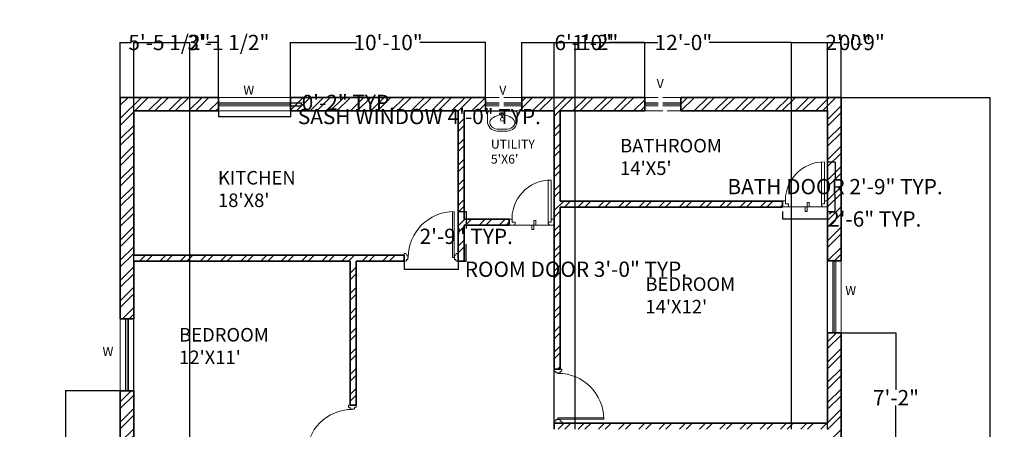
# Model space of a CAD drawing. Units: inches. Extents: x 1583 to 2239, y 1430 to 2174.
# Tile 5 of 5: x 1584 to 2239, y 1902 to 2174. Entities that reach past the tile are written whole.
import ezdxf

# ---------------------------------------------------------------- set-up
doc = ezdxf.new("R2010")
doc.units = ezdxf.units.IN
doc.linetypes.add('ACAD_ISO02W100', pattern=[15, 12, -3])
for name, color, linetype, lineweight in [('00 FURNITURE', 15, 'Continuous', 15), ('A-ANNO-DIMS', 2, 'Continuous', 18), ('A-ANNO-TEXT', 7, 'Continuous', 18), ('A-AREA-IDEN', 7, 'Continuous', 25), ('A-DOOR', 3, 'Continuous', 18), ('A-FLOR-FIXT', 9, 'Continuous', 18), ('A-GLAZ-VENT', 6, 'ACAD_ISO02W100', 13), ('A-WALL-PATT', 252, 'Continuous', 13), ('A_FUR 1', 5, 'Continuous', 5), ('WALL', 7, 'Continuous', 35), ('WINDOW', 160, 'Continuous', 18)]:
    doc.layers.add(name, color=color, linetype=linetype, lineweight=lineweight)
doc.styles.get("Standard").update_dxf_attribs({"font": 'arial.ttf'})
doc.dimstyles.get("Standard").update_dxf_attribs({"dimtxt": 10.18, "dimasz": 0.18, "dimexe": 0.18, "dimexo": 0.0625, "dimgap": 0.09, "dimtad": 0, "dimtih": 1, "dimtoh": 1, "dimdec": 0, "dimzin": 0, "dimdsep": 46, "dimlunit": 3, "dimtxsty": 'Standard', "dimcen": 0.09, "dimadec": 0, "dimazin": 0, "dimtfac": 1, "dimtdec": 0, "dimtofl": 0, "dimtmove": 0, "dimatfit": 3, "dimfxl": 1, "dimtolj": 1, "dimtzin": 0, "dimarcsym": 0})

# ---------------------------------------------------------------- blocks, each defined once
blk = doc.blocks.new('DDD')
at = {"layer": '00 FURNITURE'}
for p, q in [((-12579.77, -15859.53), (-12579.77, -15829.05)), ((-12578.77, -15859.53), (-12578.77, -15829.03)), ((-12612.02, -15857.03), (-12612.02, -15862.03)), ((-12611.02, -15857.03), (-12612.02, -15857.03)), ((-12612.02, -15862.03), (-12611.02, -15862.03)), ((-12610.52, -15858.03), (-12610.52, -15857.53)), ((-12610.52, -15861.53), (-12610.52, -15861.03)), ((-12578.77, -15859.53), (-12579.77, -15859.53)), ((-12577.52, -15858.03), (-12577.52, -15857.53)), ((-12577.52, -15861.53), (-12577.52, -15861.03)), ((-12577.02, -15857.03), (-12576.02, -15857.03)), ((-12576.02, -15862.03), (-12577.02, -15862.03)), ((-12576.02, -15857.03), (-12576.02, -15862.03))]:
    blk.add_line(p, q, dxfattribs=at)
for points in [[(-12610.52, -15861.03), (-12610.02, -15861.03, 0.414214), (-12609.52, -15860.53), (-12609.52, -15858.53, 0.414214), (-12610.02, -15858.03), (-12610.52, -15858.03)], [(-12577.52, -15861.03), (-12578.02, -15861.03, -0.414214), (-12578.52, -15860.53), (-12578.52, -15858.53, -0.414214), (-12578.02, -15858.03), (-12577.52, -15858.03)]]:
    blk.add_lwpolyline(points, format="xyb", dxfattribs=at)
for centre, radius, start, end in [((-12578.77, -15859.53), 30.5, 90, 180), ((-12611.02, -15857.53), 0.5, 0, 90), ((-12611.02, -15861.53), 0.5, 270, 0), ((-12577.02, -15857.53), 0.5, 90, 180), ((-12577.02, -15861.53), 0.5, 180, 270)]:
    blk.add_arc(centre, radius, start, end, dxfattribs=at)
blk = doc.blocks.new('ESTSET')
at = {"layer": 'A_FUR 1'}
for p, q in [((-10.44, 4.1), (-10.44, 32.1)), ((-8.44, 4.1), (-8.44, 32.1)), ((-36.44, 6.1), (-36.44, 3.1)), ((-34.44, 6.1), (-36.44, 6.1)), ((-6.44, 2.1), (-36.44, 2.1)), ((-35.44, 2.1), (-33.44, 2.1)), ((-34.44, 4.1), (-34.44, 6.1)), ((-34.44, 4.1), (-34.44, 6.1)), ((-32.44, 4.1), (-34.44, 4.1)), ((-32.44, 4.1), (-34.44, 4.1)), ((-32.44, 3.1), (-32.44, 4.1)), ((-10.44, 3.1), (-10.44, 4.1)), ((-10.44, 4.1), (-8.44, 4.1)), ((-10.44, 4.1), (-8.44, 4.1)), ((-7.44, 2.1), (-9.44, 2.1)), ((-8.44, 4.1), (-8.44, 6.1)), ((-8.44, 6.1), (-6.44, 6.1)), ((-8.44, 4.1), (-8.44, 6.1)), ((-6.44, 6.1), (-6.44, 3.1))]:
    blk.add_line(p, q, dxfattribs=at)
for points in [[(-21.44, 2.1), (-18.67, 2.1), (-18.67, 5.1), (-20.06, 5.1)], [(-21.44, 2.1), (-21.44, -0.91), (-20.06, -0.91)], [(-20.06, 5.1), (-20.06, -0.91)]]:
    blk.add_lwpolyline(points, dxfattribs=at)
for centre, radius, start, end in [((-8.91, 6.46), 25.64, 88.96059, 185.2816), ((-35.44, 3.1), 1, 180, 270), ((-33.44, 3.1), 1, 270, 0), ((-9.44, 3.1), 1, 180, 270), ((-7.44, 3.1), 1, 270, 0)]:
    blk.add_arc(centre, radius, start, end, dxfattribs=at)
blk = doc.blocks.new('s_46')
at = {"ltscale": 600}
h = blk.add_hatch(color=256, dxfattribs=at)
edge = h.paths.add_edge_path()
edge.add_line((13, 62), (14, 54))
edge.add_ellipse((4, 52), major_axis=(-10.1, 0), ratio=1, start_angle=540, end_angle=550.1755, ccw=False)
edge.add_arc((4, 52), 10.1, 270, 360, ccw=False)
edge.add_line((4, 42), (4, 41))
edge.add_line((4, 41), (12, 41))
edge.add_arc((4, 52), 13.4, 664.6981, 766.4848)
h.paths.add_polyline_path([(4, 41), (-3, 41, 0.152567), (4, 39)])
h.paths.add_polyline_path([(12, 41), (4, 41), (4, 39, 0.152567)])
h.paths.add_polyline_path([(-6, 54), (-5, 62, 0.475833), (-3, 41), (4, 41), (4, 42, -0.46724)])
for p, q in [((-6, 52), (-1, 110)), ((-6, 52), (-1, 110)), ((9, 110), (14, 54)), ((14, 52), (9, 110)), ((14, 54), (14, 52))]:
    blk.add_line(p, q, dxfattribs=at)
blk.add_lwpolyline([(-221, 171, -0.414214), (-71, 321), (79, 321, -0.414214), (229, 171), (229, 41), (209, 21), (-201, 21), (-221, 41)], format="xyb", close=True, dxfattribs=at)
blk.add_lwpolyline([(12, 75, 0.181638), (172, 142, 0.326351), (188, 223, 0.289814), (79, 291), (-71, 291, 0.289814), (-179, 223, 0.326351), (-164, 142, 0.181638), (-4, 75)], format="xyb", dxfattribs=at)
for points in [[(-17, 67), (-17, 68), (-17, 68), (-17, 68), (-18, 68), (-18, 68), (-18, 68), (-18, 68), (-18, 68), (-18, 68), (-18, 69), (-19, 69), (-19, 69), (-19, 69), (-19, 69), (-19, 69), (-19, 69), (-19, 69), (-20, 69), (-20, 69), (-20, 69), (-20, 69), (-20, 70), (-21, 70), (-21, 70), (-21, 70), (-21, 70), (-21, 70), (-21, 70), (-22, 70), (-22, 71), (-22, 71), (-22, 71), (-22, 71), (-22, 70), (-23, 70), (-23, 70), (-23, 70), (-23, 70), (-23, 70), (-24, 71), (-24, 71), (-24, 71), (-24, 71), (-24, 71), (-25, 71), (-25, 71), (-25, 71), (-25, 71), (-25, 71), (-25, 71), (-26, 71), (-26, 71), (-26, 71), (-26, 71), (-26, 71), (-27, 71), (-27, 71), (-27, 71), (-27, 71), (-27, 71), (-28, 71), (-28, 71), (-28, 71), (-28, 71), (-28, 71), (-29, 71), (-29, 70), (-29, 70), (-29, 70), (-29, 70), (-30, 70), (-30, 70), (-30, 70), (-31, 70), (-31, 70), (-31, 70), (-31, 69), (-32, 68), (-32, 68), (-33, 68), (-33, 68), (-34, 68), (-34, 68), (-34, 68), (-34, 67), (-34, 67), (-34, 67), (-34, 67), (-35, 67), (-35, 66), (-35, 66), (-35, 66), (-35, 66), (-36, 66), (-36, 66), (-36, 66), (-36, 65), (-36, 65), (-36, 65), (-36, 65), (-36, 65), (-36, 64), (-36, 64), (-36, 64), (-36, 64), (-36, 64), (-37, 64), (-37, 64), (-37, 63), (-37, 63), (-37, 63), (-37, 63), (-37, 63), (-37, 63), (-37, 62), (-37, 62), (-37, 62), (-37, 62), (-37, 62), (-37, 61), (-37, 61), (-37, 61), (-38, 61), (-38, 61), (-38, 61), (-38, 60), (-38, 60), (-38, 60), (-38, 60), (-38, 60), (-38, 59), (-37, 59), (-37, 59), (-37, 59), (-37, 59), (-37, 58), (-38, 58), (-38, 58), (-38, 58), (-38, 58), (-38, 57), (-38, 57), (-38, 57), (-38, 57), (-38, 57), (-37, 57), (-37, 56), (-37, 56), (-37, 56), (-37, 56), (-37, 56), (-37, 55), (-37, 55), (-37, 55), (-37, 55), (-37, 55), (-37, 54), (-37, 54), (-37, 54), (-37, 54), (-37, 54), (-36, 54), (-36, 54), (-36, 53), (-36, 53), (-36, 53), (-36, 53), (-36, 53), (-36, 52), (-36, 52), (-36, 52), (-36, 52), (-36, 52), (-36, 52), (-35, 51), (-35, 51), (-35, 51), (-35, 51), (-35, 51), (-34, 51), (-34, 51), (-34, 51), (-34, 51), (-34, 50), (-34, 50), (-34, 50), (-34, 50), (-34, 50), (-34, 49), (-33, 49), (-33, 49), (-33, 49), (-33, 49), (-33, 49), (-32, 49), (-32, 49), (-32, 49), (-32, 49), (-32, 49), (-32, 49), (-31, 48), (-31, 48), (-31, 48), (-31, 48), (-31, 48), (-31, 48), (-31, 48), (-30, 48), (-30, 48), (-30, 48), (-30, 48), (-30, 48), (-29, 48), (-29, 48), (-29, 47), (-29, 47), (-29, 47), (-28, 47), (-28, 47), (-28, 47), (-28, 47), (-28, 47), (-28, 47), (-27, 47), (-27, 47), (-27, 47), (-27, 47), (-27, 47), (-26, 47), (-26, 47), (-26, 47), (-26, 47), (-26, 47), (-25, 47), (-25, 47), (-25, 47), (-25, 46), (-25, 46), (-25, 47), (-24, 47), (-24, 47), (-24, 47), (-24, 47), (-24, 47), (-23, 47), (-23, 47), (-23, 47), (-23, 47), (-23, 47), (-22, 47), (-22, 47), (-22, 47), (-22, 47), (-22, 47), (-22, 47), (-21, 47), (-21, 47), (-21, 48), (-21, 48), (-21, 48), (-21, 48), (-20, 48), (-20, 48), (-20, 48), (-20, 48), (-20, 48), (-19, 48), (-19, 48), (-19, 48), (-19, 48), (-19, 48), (-19, 49), (-19, 49), (-18, 49), (-18, 49), (-18, 49), (-18, 50), (-18, 50), (-18, 50), (-18, 50), (-17, 50), (-17, 50), (-17, 50), (-17, 50), (-17, 50), (-17, 50), (-16, 50), (-16, 51), (-16, 51), (-16, 51), (-16, 51), (-16, 51), (-16, 52), (-16, 52), (-16, 52), (-16, 52), (-15, 52), (-15, 52), (-15, 52), (-15, 53), (-15, 53), (-15, 53), (-15, 53), (-15, 53), (-15, 53), (-15, 54), (-15, 54), (-15, 54), (-15, 54), (-15, 54), (-14, 55), (-14, 55), (-14, 55), (-14, 55), (-14, 55), (-14, 55), (-14, 56), (-14, 56), (-14, 56), (-14, 56), (-14, 56), (-14, 56), (-14, 57), (-14, 57), (-14, 57), (-14, 57), (-14, 57), (-14, 58), (-14, 58), (-13, 58), (-13, 58), (-13, 58), (-13, 59), (-13, 59), (-13, 59), (-13, 59), (-13, 59), (-13, 60), (-14, 60), (-14, 60), (-14, 60), (-14, 60), (-14, 60), (-14, 61), (-14, 61), (-14, 61), (-14, 61), (-14, 61), (-14, 62), (-14, 62), (-14, 62), (-14, 62), (-14, 62), (-14, 62), (-14, 63), (-14, 63), (-14, 63), (-15, 63), (-15, 63), (-15, 64), (-15, 64), (-15, 64), (-15, 64), (-15, 64), (-15, 65), (-15, 65), (-15, 65), (-15, 65), (-15, 65), (-15, 65), (-15, 65), (-16, 65), (-16, 66), (-16, 66), (-16, 66), (-16, 66), (-16, 66), (-16, 67), (-16, 67), (-16, 67), (-16, 67), (-17, 67), (-17, 67)], [(22, 61), (22, 61), (22, 61), (22, 62), (22, 62), (22, 62), (22, 62), (22, 62), (22, 62), (23, 63), (23, 63), (23, 63), (23, 63), (23, 63), (23, 64), (23, 64), (23, 64), (23, 64), (23, 64), (23, 65), (23, 65), (23, 65), (23, 65), (24, 65), (24, 65), (24, 65), (24, 65), (24, 66), (24, 66), (24, 66), (25, 66), (25, 66), (25, 67), (25, 67), (25, 67), (25, 67), (25, 67), (25, 67), (25, 67), (25, 68), (26, 68), (26, 68), (26, 68), (26, 68), (26, 68), (27, 68), (27, 68), (27, 68), (27, 69), (27, 69), (27, 69), (27, 69), (27, 69), (28, 69), (28, 69), (28, 69), (28, 69), (28, 69), (29, 69), (29, 69), (29, 70), (29, 70), (29, 70), (29, 70), (30, 70), (30, 70), (30, 70), (30, 70), (30, 71), (30, 71), (31, 71), (31, 71), (31, 70), (31, 70), (31, 70), (32, 70), (32, 70), (32, 70), (32, 71), (32, 71), (32, 71), (33, 71), (33, 71), (33, 71), (33, 71), (33, 71), (34, 71), (34, 71), (34, 71), (34, 71), (34, 71), (34, 71), (35, 71), (35, 71), (35, 71), (35, 71), (36, 71), (36, 71), (36, 71), (36, 71), (36, 71), (36, 71), (37, 71), (37, 71), (37, 71), (37, 70), (37, 70), (38, 70), (38, 70), (38, 70), (38, 70), (39, 70), (39, 70), (39, 70), (40, 70), (40, 69), (40, 68), (41, 68), (41, 68), (42, 68), (42, 68), (42, 68), (42, 68), (42, 67), (43, 67), (43, 67), (43, 67), (43, 67), (43, 66), (43, 66), (44, 66), (44, 66), (44, 66), (44, 66), (44, 66), (44, 65), (44, 65), (44, 65), (44, 65), (44, 65), (44, 64), (44, 64), (45, 64), (45, 64), (45, 64), (45, 64), (45, 64), (45, 63), (45, 63), (45, 63), (45, 63), (45, 63), (45, 63), (45, 62), (45, 62), (45, 62), (45, 62), (45, 62), (46, 61), (46, 61), (46, 61), (46, 61), (46, 61), (46, 61), (46, 60), (46, 60), (46, 60), (46, 60), (46, 60), (46, 59), (46, 59), (46, 59), (46, 59), (46, 59), (46, 58), (46, 58), (46, 58), (46, 58), (46, 58), (46, 57), (46, 57), (46, 57), (46, 57), (46, 57), (46, 57), (46, 56), (46, 56), (45, 56), (45, 56), (45, 56), (45, 55), (45, 55), (45, 55), (45, 55), (45, 55), (45, 54), (45, 54), (45, 54), (45, 54), (45, 54), (45, 54), (45, 54), (45, 53), (44, 53), (44, 53), (44, 53), (44, 53), (44, 52), (44, 52), (44, 52), (44, 52), (44, 52), (44, 52), (44, 51), (44, 51), (43, 51), (43, 51), (43, 51), (43, 51), (43, 51), (43, 51), (42, 51), (42, 50), (42, 50), (42, 50), (42, 50), (42, 50), (42, 49), (42, 49), (42, 49), (41, 49), (41, 49), (41, 49), (41, 49), (41, 49), (40, 49), (40, 49), (40, 49), (40, 49), (40, 48), (40, 48), (40, 48), (39, 48), (39, 48), (39, 48), (39, 48), (39, 48), (39, 48), (38, 48), (38, 48), (38, 48), (38, 48), (38, 48), (37, 47), (37, 47), (37, 47), (37, 47), (37, 47), (37, 47), (36, 47), (36, 47), (36, 47), (36, 47), (36, 47), (36, 47), (35, 47), (35, 47), (35, 47), (35, 47), (34, 47), (34, 47), (34, 47), (34, 47), (34, 47), (34, 47), (33, 46), (33, 46), (33, 47), (33, 47), (33, 47), (32, 47), (32, 47), (32, 47), (32, 47), (32, 47), (32, 47), (31, 47), (31, 47), (31, 47), (31, 47), (31, 47), (30, 47), (30, 47), (30, 47), (30, 47), (30, 47), (30, 48), (29, 48), (29, 48), (29, 48), (29, 48), (29, 48), (29, 48), (28, 48), (28, 48), (28, 48), (28, 48), (28, 48), (27, 48), (27, 48), (27, 49), (27, 49), (27, 49), (27, 49), (27, 49), (27, 50), (26, 50), (26, 50), (26, 50), (26, 50), (26, 50), (25, 50), (25, 50), (25, 50), (25, 50), (25, 50), (25, 51), (25, 51), (25, 51), (25, 51), (25, 51), (24, 52), (24, 52), (24, 52), (24, 52), (24, 52), (24, 52), (24, 52), (23, 53), (23, 53), (23, 53), (23, 53), (23, 53), (23, 53), (23, 54), (23, 54), (23, 54), (23, 54), (23, 54), (23, 55), (23, 55), (23, 55), (22, 55), (22, 55), (22, 55), (22, 56), (22, 56), (22, 56), (22, 56), (22, 56), (22, 56), (22, 57), (22, 57), (22, 57), (22, 57), (22, 57), (22, 58), (22, 58), (22, 58), (22, 58), (22, 58), (22, 59), (22, 59), (22, 59), (22, 59), (22, 59), (22, 60), (22, 60), (22, 60), (22, 60), (22, 60), (22, 60), (22, 61), (22, 61)]]:
    blk.add_lwpolyline(points, close=True, dxfattribs=at)
blk.add_circle((4, 146), 28, dxfattribs=at)
for centre, radius, start, end in [((4, 52), 10.1, 169.8245, 0), ((4, 108), 5.42, 24.6783, 155.3217)]:
    blk.add_arc(centre, radius, start, end, dxfattribs=at)
for centre, major_axis, ratio, start_param, end_param in [((4, 52), (-10.1, 0), 1, 6.10559, 9.602373), ((4, 110), (-4.93, 0), 0.641024, 3.141593, 6.283185)]:
    blk.add_ellipse(centre, major_axis=major_axis, ratio=ratio, start_param=start_param, end_param=end_param, dxfattribs=at)
blk = doc.blocks.new('*D10')
at = {"layer": 'A-ANNO-DIMS', "color": 0, "lineweight": -2, "transparency": 16777216}
for p, q in [((2130.59, 2122.64), (2229.81, 2122.64)), ((2229.63, 2122.46), (2229.63, 1827.93)), ((2229.63, 1522.82), (2229.63, 1817.35)), ((2130.59, 1522.64), (2229.81, 1522.64))]:
    blk.add_line(p, q, dxfattribs=at)
at = {"layer": 'A-ANNO-DIMS', "color": 0, "transparency": 16777216}
for points in [[(2229.6, 2122.46), (2229.66, 2122.46), (2229.63, 2122.64)], [(2229.6, 1522.82), (2229.66, 1522.82), (2229.63, 1522.64)]]:
    blk.add_solid(points, dxfattribs=at)
at = {"layer": 'Defpoints', "color": 0, "transparency": 16777216}
for p in [(2130.53, 2122.64), (2130.53, 1522.64), (2229.63, 1522.64)]:
    blk.add_point(p, dxfattribs=at)
at = {"layer": 'A-ANNO-DIMS', "color": 0, "transparency": 16777216, "insert": (2229.63, 1822.64), "char_height": 10.18, "attachment_point": 5}
blk.add_mtext("\\A1;50'", dxfattribs=at)
blk = doc.blocks.new('WIN-SASH-48IN')
for p, q in [((48, 2), (0, 2)), ((48, 1), (0, 1)), ((48, 0), (0, 0))]:
    blk.add_line(p, q)
blk = doc.blocks.new('VENT-GRILLE-24IN')
for p, q in [((24, 2), (0, 2)), ((24, 1), (0, 1)), ((24, 0), (0, 0))]:
    blk.add_line(p, q)
blk = doc.blocks.new('*D13')
at = {"layer": 'A-ANNO-DIMS', "color": 0, "lineweight": -2, "transparency": 16777216}
for p, q in [((1715.9, 2117.08), (1715.9, 2109.76)), ((1763.9, 2117.08), (1763.9, 2109.76)), ((1716.08, 2109.94), (1763.72, 2109.94)), ((1763.9, 2109.94), (1764.08, 2109.94))]:
    blk.add_line(p, q, dxfattribs=at)
at = {"layer": 'A-ANNO-DIMS', "color": 0, "transparency": 16777216}
for points in [[(1716.08, 2109.97), (1716.08, 2109.91), (1715.9, 2109.94)], [(1763.72, 2109.97), (1763.72, 2109.91), (1763.9, 2109.94)]]:
    blk.add_solid(points, dxfattribs=at)
at = {"layer": 'Defpoints', "color": 0, "transparency": 16777216}
for p in [(1715.9, 2117.14), (1763.9, 2117.14), (1763.9, 2109.94)]:
    blk.add_point(p, dxfattribs=at)
at = {"layer": 'A-ANNO-DIMS', "color": 0, "transparency": 16777216, "insert": (1849.69, 2109.94), "char_height": 10.18, "attachment_point": 5}
blk.add_mtext('\\A1;SASH WINDOW 4\'-0" TYP.', dxfattribs=at)
blk = doc.blocks.new('*D14')
at = {"layer": 'A-ANNO-DIMS', "color": 0, "lineweight": -2, "transparency": 16777216}
for p, q in [((1763.97, 2119.14), (1771.28, 2119.14)), ((1771.1, 2119.14), (1771.1, 2119.32)), ((1771.1, 2119.32), (1771.28, 2119.32)), ((1771.1, 2117.32), (1771.1, 2118.96)), ((1763.97, 2117.14), (1771.28, 2117.14))]:
    blk.add_line(p, q, dxfattribs=at)
at = {"layer": 'A-ANNO-DIMS', "color": 0, "transparency": 16777216}
for points in [[(1771.07, 2118.96), (1771.13, 2118.96), (1771.1, 2119.14)], [(1771.07, 2117.32), (1771.13, 2117.32), (1771.1, 2117.14)]]:
    blk.add_solid(points, dxfattribs=at)
at = {"layer": 'Defpoints', "color": 0, "transparency": 16777216}
for p in [(1763.9, 2119.14), (1771.1, 2119.14), (1763.9, 2117.14)]:
    blk.add_point(p, dxfattribs=at)
at = {"layer": 'A-ANNO-DIMS', "color": 0, "transparency": 16777216, "insert": (1802.4, 2119.32), "char_height": 10.18, "attachment_point": 5}
blk.add_mtext('\\A1;0\'-2" TYP.', dxfattribs=at)
blk = doc.blocks.new('*D17')
at = {"layer": 'A-ANNO-DIMS', "color": 0, "lineweight": -2, "transparency": 16777216}
for p, q in [((1839.53, 2013.58), (1839.53, 2008.06)), ((1875.53, 2013.58), (1875.53, 2008.06)), ((1839.71, 2008.24), (1875.35, 2008.24)), ((1875.53, 2008.24), (1875.71, 2008.24))]:
    blk.add_line(p, q, dxfattribs=at)
at = {"layer": 'A-ANNO-DIMS', "color": 0, "transparency": 16777216}
for points in [[(1839.71, 2008.27), (1839.71, 2008.21), (1839.53, 2008.24)], [(1875.35, 2008.27), (1875.35, 2008.21), (1875.53, 2008.24)]]:
    blk.add_solid(points, dxfattribs=at)
at = {"layer": 'Defpoints', "color": 0, "transparency": 16777216}
for p in [(1839.53, 2013.64), (1875.53, 2013.64), (1875.53, 2008.24)]:
    blk.add_point(p, dxfattribs=at)
at = {"layer": 'A-ANNO-DIMS', "color": 0, "transparency": 16777216, "insert": (1953.97, 2008.24), "char_height": 10.18, "attachment_point": 5}
blk.add_mtext('\\A1;ROOM DOOR 3\'-0" TYP.', dxfattribs=at)
blk = doc.blocks.new('*D18')
at = {"layer": 'A-ANNO-DIMS', "color": 0, "lineweight": -2, "transparency": 16777216}
for p, q in [((1875.59, 2046.64), (1881.11, 2046.64)), ((1880.93, 2046.46), (1880.93, 2035.43)), ((1880.93, 2013.82), (1880.93, 2024.85)), ((1875.59, 2013.64), (1881.11, 2013.64))]:
    blk.add_line(p, q, dxfattribs=at)
at = {"layer": 'A-ANNO-DIMS', "color": 0, "transparency": 16777216}
for points in [[(1880.9, 2046.46), (1880.96, 2046.46), (1880.93, 2046.64)], [(1880.9, 2013.82), (1880.96, 2013.82), (1880.93, 2013.64)]]:
    blk.add_solid(points, dxfattribs=at)
at = {"layer": 'Defpoints', "color": 0, "transparency": 16777216}
for p in [(1875.53, 2046.64), (1880.93, 2046.64), (1875.53, 2013.64)]:
    blk.add_point(p, dxfattribs=at)
at = {"layer": 'A-ANNO-DIMS', "color": 0, "transparency": 16777216, "insert": (1880.93, 2030.14), "char_height": 10.18, "attachment_point": 5}
blk.add_mtext('\\A1;2\'-9" TYP.', dxfattribs=at)
blk = doc.blocks.new('*D19')
at = {"layer": 'A-ANNO-DIMS', "color": 0, "lineweight": -2, "transparency": 16777216}
for p, q in [((2121.64, 2079.82), (2126.72, 2079.82)), ((2126.54, 2079.64), (2126.54, 2068.61)), ((2126.54, 2046.86), (2126.54, 2057.9)), ((2121.64, 2046.68), (2126.72, 2046.68))]:
    blk.add_line(p, q, dxfattribs=at)
at = {"layer": 'A-ANNO-DIMS', "color": 0, "transparency": 16777216}
for points in [[(2126.51, 2079.64), (2126.57, 2079.64), (2126.54, 2079.82)], [(2126.51, 2046.86), (2126.57, 2046.86), (2126.54, 2046.68)]]:
    blk.add_solid(points, dxfattribs=at)
at = {"layer": 'Defpoints', "color": 0, "transparency": 16777216}
for p in [(2121.57, 2079.82), (2126.54, 2079.82), (2121.57, 2046.68)]:
    blk.add_point(p, dxfattribs=at)
at = {"layer": 'A-ANNO-DIMS', "color": 0, "transparency": 16777216, "insert": (2126.54, 2063.25), "char_height": 10.18, "attachment_point": 5}
blk.add_mtext('\\A1;BATH DOOR 2\'-9" TYP.', dxfattribs=at)
blk = doc.blocks.new('*D20')
at = {"layer": 'A-ANNO-DIMS', "color": 0, "lineweight": -2, "transparency": 16777216}
for p, q in [((2091.57, 2046.62), (2091.57, 2041.53)), ((2121.57, 2046.62), (2121.57, 2041.53)), ((2091.75, 2041.71), (2121.39, 2041.71)), ((2121.57, 2041.71), (2121.75, 2041.71))]:
    blk.add_line(p, q, dxfattribs=at)
at = {"layer": 'A-ANNO-DIMS', "color": 0, "transparency": 16777216}
for points in [[(2091.75, 2041.74), (2091.75, 2041.68), (2091.57, 2041.71)], [(2121.39, 2041.74), (2121.39, 2041.68), (2121.57, 2041.71)]]:
    blk.add_solid(points, dxfattribs=at)
at = {"layer": 'Defpoints', "color": 0, "transparency": 16777216}
for p in [(2091.57, 2046.68), (2121.57, 2046.68), (2121.57, 2041.71)]:
    blk.add_point(p, dxfattribs=at)
at = {"layer": 'A-ANNO-DIMS', "color": 0, "transparency": 16777216, "insert": (2152.96, 2041.71), "char_height": 10.18, "attachment_point": 5}
blk.add_mtext('\\A1;2\'-6" TYP.', dxfattribs=at)
blk = doc.blocks.new('*D29')
at = {"layer": 'A-ANNO-DIMS', "color": 0, "lineweight": -2, "transparency": 16777216}
for p, q in [((1650.53, 2122.7), (1650.53, 2159.42)), ((1650.71, 2159.24), (1657.74, 2159.24)), ((1715.72, 2159.24), (1708.7, 2159.24)), ((1715.9, 2122.7), (1715.9, 2159.42))]:
    blk.add_line(p, q, dxfattribs=at)
at = {"layer": 'A-ANNO-DIMS', "color": 0, "transparency": 16777216}
for points in [[(1650.71, 2159.27), (1650.71, 2159.21), (1650.53, 2159.24)], [(1715.72, 2159.27), (1715.72, 2159.21), (1715.9, 2159.24)]]:
    blk.add_solid(points, dxfattribs=at)
at = {"layer": 'Defpoints', "color": 0, "transparency": 16777216}
for p in [(1715.9, 2159.24), (1650.53, 2122.64), (1715.9, 2122.64)]:
    blk.add_point(p, dxfattribs=at)
at = {"layer": 'A-ANNO-DIMS', "color": 0, "transparency": 16777216, "insert": (1683.22, 2159.24), "char_height": 10.18, "attachment_point": 5}
blk.add_mtext('\\A1;5\'-5 1/2"', dxfattribs=at)
blk = doc.blocks.new('*D30')
at = {"layer": 'A-ANNO-DIMS', "color": 0, "lineweight": -2, "transparency": 16777216}
for p, q in [((1763.9, 2122.7), (1763.9, 2159.42)), ((1764.08, 2159.24), (1807.83, 2159.24)), ((1893.68, 2159.24), (1849.93, 2159.24)), ((1893.86, 2122.7), (1893.86, 2159.42))]:
    blk.add_line(p, q, dxfattribs=at)
at = {"layer": 'A-ANNO-DIMS', "color": 0, "transparency": 16777216}
for points in [[(1764.08, 2159.27), (1764.08, 2159.21), (1763.9, 2159.24)], [(1893.68, 2159.27), (1893.68, 2159.21), (1893.86, 2159.24)]]:
    blk.add_solid(points, dxfattribs=at)
at = {"layer": 'Defpoints', "color": 0, "transparency": 16777216}
for p in [(1893.86, 2159.24), (1763.9, 2122.64), (1893.86, 2122.64)]:
    blk.add_point(p, dxfattribs=at)
at = {"layer": 'A-ANNO-DIMS', "color": 0, "transparency": 16777216, "insert": (1828.88, 2159.24), "char_height": 10.18, "attachment_point": 5}
blk.add_mtext('\\A1;10\'-10"', dxfattribs=at)
blk = doc.blocks.new('*D31')
at = {"layer": 'A-ANNO-DIMS', "color": 0, "lineweight": -2, "transparency": 16777216}
for p, q in [((1917.86, 2122.7), (1917.86, 2159.42)), ((1918.04, 2159.24), (1941.23, 2159.24)), ((1999.62, 2159.24), (1976.43, 2159.24)), ((1999.8, 2122.7), (1999.8, 2159.42))]:
    blk.add_line(p, q, dxfattribs=at)
at = {"layer": 'A-ANNO-DIMS', "color": 0, "transparency": 16777216}
for points in [[(1918.04, 2159.27), (1918.04, 2159.21), (1917.86, 2159.24)], [(1999.62, 2159.27), (1999.62, 2159.21), (1999.8, 2159.24)]]:
    blk.add_solid(points, dxfattribs=at)
at = {"layer": 'Defpoints', "color": 0, "transparency": 16777216}
for p in [(1999.8, 2159.24), (1917.86, 2122.64), (1999.8, 2122.64)]:
    blk.add_point(p, dxfattribs=at)
at = {"layer": 'A-ANNO-DIMS', "color": 0, "transparency": 16777216, "insert": (1958.83, 2159.24), "char_height": 10.18, "attachment_point": 5}
blk.add_mtext('\\A1;6\'-10"', dxfattribs=at)
blk = doc.blocks.new('*D39')
at = {"layer": 'A-ANNO-DIMS', "color": 0, "lineweight": -2, "transparency": 16777216}
for p, q in [((1650.47, 1927.26), (1613.75, 1927.26)), ((1613.93, 1927.08), (1613.93, 1890.96)), ((1613.93, 1844.13), (1613.93, 1880.25)), ((1650.47, 1843.95), (1613.75, 1843.95))]:
    blk.add_line(p, q, dxfattribs=at)
at = {"layer": 'A-ANNO-DIMS', "color": 0, "transparency": 16777216}
for points in [[(1613.9, 1927.08), (1613.96, 1927.08), (1613.93, 1927.26)], [(1613.9, 1844.13), (1613.96, 1844.13), (1613.93, 1843.95)]]:
    blk.add_solid(points, dxfattribs=at)
at = {"layer": 'Defpoints', "color": 0, "transparency": 16777216}
for p in [(1613.93, 1927.26), (1650.53, 1927.26), (1650.53, 1843.95)]:
    blk.add_point(p, dxfattribs=at)
at = {"layer": 'A-ANNO-DIMS', "color": 0, "transparency": 16777216, "insert": (1613.93, 1885.6), "char_height": 10.18, "attachment_point": 5}
blk.add_mtext('\\A1;6\'-11 1/2"', dxfattribs=at)
blk = doc.blocks.new('*D43')
at = {"layer": 'A-ANNO-DIMS', "color": 0, "lineweight": -2, "transparency": 16777216}
for p, q in [((2130.59, 1965.82), (2167.31, 1965.82)), ((2167.13, 1965.64), (2167.13, 1927.92)), ((2167.13, 1879.81), (2167.13, 1917.52)), ((2130.59, 1879.63), (2167.31, 1879.63))]:
    blk.add_line(p, q, dxfattribs=at)
at = {"layer": 'A-ANNO-DIMS', "color": 0, "transparency": 16777216}
for points in [[(2167.1, 1965.64), (2167.16, 1965.64), (2167.13, 1965.82)], [(2167.1, 1879.81), (2167.16, 1879.81), (2167.13, 1879.63)]]:
    blk.add_solid(points, dxfattribs=at)
at = {"layer": 'Defpoints', "color": 0, "transparency": 16777216}
for p in [(2130.53, 1965.82), (2167.13, 1965.82), (2130.53, 1879.63)]:
    blk.add_point(p, dxfattribs=at)
at = {"layer": 'A-ANNO-DIMS', "color": 0, "transparency": 16777216, "insert": (2167.13, 1922.72), "char_height": 10.18, "attachment_point": 5}
blk.add_mtext('\\A1;7\'-2"', dxfattribs=at)
blk = doc.blocks.new('*D46')
at = {"layer": 'A-ANNO-DIMS', "color": 0, "lineweight": -2, "transparency": 16777216}
for p, q in [((1953.53, 1901.7), (1953.53, 2159.42)), ((1953.71, 2159.24), (2008.44, 2159.24)), ((2097.35, 2159.24), (2042.63, 2159.24)), ((2097.53, 1901.7), (2097.53, 2159.42))]:
    blk.add_line(p, q, dxfattribs=at)
at = {"layer": 'A-ANNO-DIMS', "color": 0, "transparency": 16777216}
for points in [[(1953.71, 2159.27), (1953.71, 2159.21), (1953.53, 2159.24)], [(2097.35, 2159.27), (2097.35, 2159.21), (2097.53, 2159.24)]]:
    blk.add_solid(points, dxfattribs=at)
at = {"layer": 'Defpoints', "color": 0, "transparency": 16777216}
for p in [(2097.53, 2159.24), (1953.53, 1901.64), (2097.53, 1901.64)]:
    blk.add_point(p, dxfattribs=at)
at = {"layer": 'A-ANNO-DIMS', "color": 0, "transparency": 16777216, "insert": (2025.53, 2159.24), "char_height": 10.18, "attachment_point": 5}
blk.add_mtext('\\A1;12\'-0"', dxfattribs=at)
blk = doc.blocks.new('*D48')
at = {"layer": 'A-ANNO-DIMS', "color": 0, "lineweight": -2, "transparency": 16777216}
for p, q in [((2097.53, 1901.7), (2097.53, 2159.42)), ((2097.71, 2159.24), (2121.35, 2159.24)), ((2121.53, 1901.7), (2121.53, 2159.42)), ((2121.53, 2159.24), (2121.71, 2159.24))]:
    blk.add_line(p, q, dxfattribs=at)
at = {"layer": 'A-ANNO-DIMS', "color": 0, "transparency": 16777216}
for points in [[(2097.71, 2159.27), (2097.71, 2159.21), (2097.53, 2159.24)], [(2121.35, 2159.27), (2121.35, 2159.21), (2121.53, 2159.24)]]:
    blk.add_solid(points, dxfattribs=at)
at = {"layer": 'Defpoints', "color": 0, "transparency": 16777216}
for p in [(2121.53, 2159.24), (2097.53, 1901.64), (2121.53, 1901.64)]:
    blk.add_point(p, dxfattribs=at)
at = {"layer": 'A-ANNO-DIMS', "color": 0, "transparency": 16777216, "insert": (2135.42, 2159.24), "char_height": 10.18, "attachment_point": 5}
blk.add_mtext('\\A1;2\'-0"', dxfattribs=at)
blk = doc.blocks.new('*D50')
at = {"layer": 'A-ANNO-DIMS', "color": 0, "lineweight": -2, "transparency": 16777216}
for p, q in [((2121.53, 2113.7), (2121.53, 2159.42)), ((2121.71, 2159.24), (2130.35, 2159.24)), ((2130.53, 2122.7), (2130.53, 2159.42)), ((2130.53, 2159.24), (2130.71, 2159.24))]:
    blk.add_line(p, q, dxfattribs=at)
at = {"layer": 'A-ANNO-DIMS', "color": 0, "transparency": 16777216}
for points in [[(2121.71, 2159.27), (2121.71, 2159.21), (2121.53, 2159.24)], [(2130.35, 2159.27), (2130.35, 2159.21), (2130.53, 2159.24)]]:
    blk.add_solid(points, dxfattribs=at)
at = {"layer": 'Defpoints', "color": 0, "transparency": 16777216}
for p in [(2130.53, 2159.24), (2130.53, 2122.64), (2121.53, 2113.64)]:
    blk.add_point(p, dxfattribs=at)
at = {"layer": 'A-ANNO-DIMS', "color": 0, "transparency": 16777216, "insert": (2144.33, 2159.24), "char_height": 10.18, "attachment_point": 5}
blk.add_mtext('\\A1;0\'-9"', dxfattribs=at)
blk = doc.blocks.new('*D55')
at = {"layer": 'A-ANNO-DIMS', "color": 0, "lineweight": -2, "transparency": 16777216}
for p, q in [((1659.53, 1877.7), (1659.53, 2159.42)), ((1659.71, 2159.24), (1696.67, 2159.24)), ((1696.85, 1877.57), (1696.85, 2159.42)), ((1696.85, 2159.24), (1697.03, 2159.24))]:
    blk.add_line(p, q, dxfattribs=at)
at = {"layer": 'A-ANNO-DIMS', "color": 0, "transparency": 16777216}
for points in [[(1659.71, 2159.27), (1659.71, 2159.21), (1659.53, 2159.24)], [(1696.67, 2159.27), (1696.67, 2159.21), (1696.85, 2159.24)]]:
    blk.add_solid(points, dxfattribs=at)
at = {"layer": 'Defpoints', "color": 0, "transparency": 16777216}
for p in [(1696.85, 2159.24), (1659.53, 1877.64), (1696.85, 1877.51)]:
    blk.add_point(p, dxfattribs=at)
at = {"layer": 'A-ANNO-DIMS', "color": 0, "transparency": 16777216, "insert": (1722.51, 2159.24), "char_height": 10.18, "attachment_point": 5}
blk.add_mtext('\\A1;3\'-1 1/2"', dxfattribs=at)
blk = doc.blocks.new('*D58')
at = {"layer": 'A-ANNO-DIMS', "color": 0, "lineweight": -2, "transparency": 16777216}
for p, q in [((1939.53, 1901.7), (1939.53, 2159.42)), ((1939.71, 2159.24), (1953.35, 2159.24)), ((1953.53, 1901.7), (1953.53, 2159.42)), ((1953.53, 2159.24), (1953.71, 2159.24))]:
    blk.add_line(p, q, dxfattribs=at)
at = {"layer": 'A-ANNO-DIMS', "color": 0, "transparency": 16777216}
for points in [[(1939.71, 2159.27), (1939.71, 2159.21), (1939.53, 2159.24)], [(1953.35, 2159.27), (1953.35, 2159.21), (1953.53, 2159.24)]]:
    blk.add_solid(points, dxfattribs=at)
at = {"layer": 'Defpoints', "color": 0, "transparency": 16777216}
for p in [(1953.53, 2159.24), (1939.53, 1901.64), (1953.53, 1901.64)]:
    blk.add_point(p, dxfattribs=at)
at = {"layer": 'A-ANNO-DIMS', "color": 0, "transparency": 16777216, "insert": (1966.85, 2159.24), "char_height": 10.18, "attachment_point": 5}
blk.add_mtext('\\A1;1\'-2"', dxfattribs=at)

msp = doc.modelspace()

# ---------------------------------------------------------------- hatches: boundary and pattern name
at = {"layer": 'A-WALL-PATT'}
h = msp.add_hatch(dxfattribs=at)
h.set_pattern_fill('ANSI32', color=256)
h.paths.add_polyline_path([(1715.9, 2122.64), (1650.53, 2122.64), (1650.53, 1975.26), (1659.53, 1975.26), (1659.53, 1975.26), (1659.53, 2013.64), (1803.53, 2013.64), (1803.53, 1917.64), (1807.53, 1917.64), (1807.53, 2013.64), (1839.53, 2013.64), (1839.53, 2017.64), (1659.53, 2017.64), (1659.53, 2113.64), (1715.9, 2113.64)])
h.paths.add_polyline_path([(1893.86, 2122.64), (1763.9, 2122.64), (1763.9, 2113.64), (1875.53, 2113.64), (1875.53, 2013.64), (1879.53, 2013.64), (1879.53, 2037.64), (1909.53, 2037.64), (1909.53, 2041.64), (1879.53, 2041.64), (1879.53, 2113.64), (1893.86, 2113.64)])
h.paths.add_polyline_path([(1999.8, 2122.64), (1917.86, 2122.64), (1917.86, 2113.64), (1939.53, 2113.64), (1939.53, 2037.64), (1939.53, 1941.64), (1943.53, 1941.64), (1943.53, 2049.64), (2091.53, 2049.64), (2091.53, 2053.64), (1943.53, 2053.64), (1943.53, 2113.64), (1999.8, 2113.64)])
h.paths.add_polyline_path([(2130.53, 2122.64), (2023.8, 2122.64), (2023.8, 2113.64), (2121.53, 2113.64), (2121.53, 2049.64), (2121.53, 2013.82), (2130.53, 2013.82), (2130.53, 2013.82)])
h.paths.add_polyline_path([(2130.53, 1965.82), (2121.53, 1965.82), (2121.53, 1905.64), (1944.53, 1905.64), (1944.53, 1905.64), (1939.53, 1905.64), (1939.53, 1901.64), (2121.53, 1901.64), (2121.53, 1879.63), (2130.53, 1879.63)])
h.paths.add_polyline_path([(2130.53, 1855.63), (2121.53, 1855.63), (2121.53, 1817.64), (1939.53, 1817.64), (1939.53, 1729.64), (1943.53, 1729.64), (1943.53, 1813.64), (2121.53, 1813.64), (2121.53, 1780.2), (2130.53, 1780.2), (2130.53, 1780.2)])
h.paths.add_polyline_path([(2130.53, 1732.2), (2121.53, 1732.2), (2121.53, 1693.64), (1944.53, 1693.64), (1944.53, 1693.64), (1939.53, 1693.64), (1900.39, 1693.64), (1900.39, 1689.64), (2121.53, 1689.64), (2121.53, 1649.31), (2130.53, 1649.31), (2130.53, 1649.31)])
h.paths.add_polyline_path([(2130.53, 1601.31), (2121.53, 1601.31), (2121.53, 1531.64), (2056.46, 1531.64), (2056.46, 1522.64), (2130.53, 1522.64)])
h.paths.add_polyline_path([(2032.46, 1531.64), (1943.39, 1531.64), (1943.39, 1526.25), (1943.39, 1526.25), (1943.39, 1522.64), (2032.46, 1522.64)])
h.paths.add_polyline_path([(1895.39, 1531.64), (1871.02, 1531.64), (1871.02, 1522.64), (1895.39, 1522.64)])
h.paths.add_polyline_path([(1847.02, 1531.64), (1807.53, 1531.64), (1807.53, 1653.64), (1803.53, 1653.64), (1803.53, 1531.64), (1750.06, 1531.64), (1750.06, 1522.64), (1847.02, 1522.64)])
h.paths.add_polyline_path([(1702.06, 1531.64), (1659.53, 1531.64), (1659.53, 1587.56), (1650.53, 1587.56), (1650.53, 1522.64), (1702.06, 1522.64)])
h.paths.add_polyline_path([(1659.53, 1927.26), (1650.53, 1927.26), (1650.53, 1843.95), (1659.53, 1843.95), (1659.53, 1877.64)])
h.paths.add_polyline_path([(1659.53, 1801.64), (1807.53, 1801.64), (1807.53, 1881.64), (1689.53, 1881.64), (1689.53, 1877.64), (1803.53, 1877.64), (1803.53, 1805.64), (1659.53, 1805.64), (1659.53, 1819.95), (1650.53, 1819.95), (1650.53, 1766.08), (1659.53, 1766.08)])
h.paths.add_polyline_path([(1659.53, 1742.08), (1650.53, 1742.08), (1650.53, 1635.56), (1659.53, 1635.56), (1659.53, 1635.56), (1659.53, 1689.64), (1807.53, 1689.64), (1840.39, 1689.64), (1840.39, 1693.64), (1807.53, 1693.64), (1807.53, 1771.64), (1803.53, 1771.64), (1803.53, 1693.64), (1786.54, 1693.64), (1786.54, 1693.64), (1768.55, 1693.64), (1659.53, 1693.64), (1659.53, 1701.64)])

# ---------------------------------------------------------------- linework, layer by layer
at = {"layer": 'A-GLAZ-VENT'}
for points in [[(1893.86, 2122.64), (1893.86, 2113.64), (1917.86, 2113.64), (1917.86, 2122.64)], [(1999.8, 2122.64), (1999.8, 2113.64), (2023.8, 2113.64), (2023.8, 2122.64)]]:
    msp.add_lwpolyline(points, close=True, dxfattribs=at)
at = {"layer": 'WALL'}
for p, q in [((1650.53, 2122.64), (1715.9, 2122.64)), ((1650.53, 1975.26), (1650.53, 2122.64)), ((1715.9, 2113.64), (1715.9, 2122.64)), ((1763.9, 2113.64), (1763.9, 2122.64)), ((1763.9, 2122.64), (1893.86, 2122.64)), ((1893.86, 2113.64), (1893.86, 2122.64)), ((1917.86, 2113.64), (1917.86, 2122.64)), ((1917.86, 2122.64), (1999.8, 2122.64)), ((1999.8, 2113.64), (1999.8, 2122.64)), ((2023.8, 2113.64), (2023.8, 2122.64)), ((2023.8, 2122.64), (2130.53, 2122.64)), ((2130.53, 2122.64), (2130.53, 2013.82)), ((1659.53, 2113.64), (1715.9, 2113.64)), ((1659.53, 2017.64), (1659.53, 2113.64)), ((1763.9, 2113.64), (1875.53, 2113.64)), ((1875.53, 2013.64), (1875.53, 2113.64)), ((1879.53, 2113.64), (1893.86, 2113.64)), ((1879.53, 2041.64), (1879.53, 2113.64)), ((1917.86, 2113.64), (1939.53, 2113.64)), ((1939.53, 2037.64), (1939.53, 2113.64)), ((1943.53, 2113.64), (1999.8, 2113.64)), ((1943.53, 2053.64), (1943.53, 2113.64)), ((2023.8, 2113.64), (2121.53, 2113.64)), ((2121.53, 2113.64), (2121.53, 2049.64)), ((1943.53, 2053.64), (2091.53, 2053.64)), ((2091.53, 2053.64), (2091.53, 2049.64)), ((1943.53, 2049.64), (2091.53, 2049.64)), ((1943.53, 1941.64), (1943.53, 2049.64)), ((2121.53, 2049.64), (2121.53, 2013.82)), ((1879.53, 2041.64), (1909.53, 2041.64)), ((1909.53, 2037.64), (1909.53, 2041.64)), ((1879.53, 2037.64), (1909.53, 2037.64)), ((1879.53, 2013.64), (1879.53, 2037.64)), ((1939.53, 1941.64), (1939.53, 2037.64)), ((1659.53, 2017.64), (1839.53, 2017.64)), ((1659.53, 2013.64), (1803.53, 2013.64)), ((1659.53, 1975.26), (1659.53, 2013.64)), ((1803.53, 1917.64), (1803.53, 2013.64)), ((1807.53, 2013.64), (1839.53, 2013.64)), ((1807.53, 1917.64), (1807.53, 2013.64)), ((1839.53, 2013.64), (1839.53, 2017.64)), ((1875.53, 2013.64), (1879.53, 2013.64)), ((2121.53, 2013.82), (2130.53, 2013.82)), ((1650.53, 1975.26), (1659.53, 1975.26)), ((2121.53, 1965.82), (2130.53, 1965.82)), ((2121.53, 1965.82), (2121.53, 1905.64)), ((2130.53, 1965.82), (2130.53, 1879.63)), ((1939.53, 1941.64), (1943.53, 1941.64)), ((1650.53, 1927.26), (1659.53, 1927.26)), ((1650.53, 1843.95), (1650.53, 1927.26)), ((1659.53, 1877.64), (1659.53, 1927.26)), ((1803.53, 1917.64), (1807.53, 1917.64)), ((1939.53, 1905.64), (2121.53, 1905.64)), ((1939.53, 1901.64), (1939.53, 1905.64))]:
    msp.add_line(p, q, dxfattribs=at)
at = {"layer": 'WINDOW'}
for p, q in [((1763.9, 2122.64), (1715.9, 2122.64)), ((1715.9, 2113.64), (1763.9, 2113.64)), ((2121.53, 2013.82), (2121.53, 1965.82)), ((2130.53, 1965.82), (2130.53, 2013.82)), ((1650.53, 1975.26), (1650.53, 1927.26)), ((1659.53, 1927.26), (1659.53, 1975.26))]:
    msp.add_line(p, q, dxfattribs=at)

# ---------------------------------------------------------------- block references
at = {"layer": 'A-DOOR'}
for name, p in [('ESTSET', (2128.02, 2047.59)), ('ESTSET', (1945.98, 2035.54)), ('DDD', (14451.56, 17875.67))]:
    msp.add_blockref(name, p, dxfattribs=at)
at = {"layer": 'A-DOOR', "rotation": 270}
msp.add_blockref('DDD', (17801.56, -10670.38), dxfattribs=at)
at = {"layer": 'A-DOOR', "xscale": -1, "rotation": 90}
msp.add_blockref('DDD', (-14054.5, -10694.38), dxfattribs=at)
at = {"layer": 'A-FLOR-FIXT', "xscale": -0.0438792252617072, "yscale": 0.0438792252617072, "zscale": 0.0438792252617072, "rotation": 180}
msp.add_blockref('s_46', (1904.71, 2114.38), dxfattribs=at)
at = {"layer": 'A-GLAZ-VENT'}
for p in [(1893.86, 2117.14), (1999.8, 2117.14)]:
    msp.add_blockref('VENT-GRILLE-24IN', p, dxfattribs=at)
at = {"layer": 'WINDOW'}
msp.add_blockref('WIN-SASH-48IN', (1715.9, 2117.14), dxfattribs=at)
for p, rotation in [((2125.03, 2013.82), 270.0000000000021), ((1654.03, 1975.26), 270.0000000000006)]:
    msp.add_blockref('WIN-SASH-48IN', p, dxfattribs=dict(at, rotation=rotation))

# ---------------------------------------------------------------- texts
at = {"layer": 'A-ANNO-TEXT', "char_height": 6, "attachment_point": 1}
for s, insert in [('V', (2007.77, 2134.91)), ('W', (1732.51, 2130.48)), ('V', (1902.9, 2130.46)), ('W', (2133.38, 1997.01)), ('W', (1638.71, 1956.42))]:
    msp.add_mtext_dynamic_manual_height_columns(s, width=236.3031, gutter_width=12.5, heights=[0], dxfattribs=dict(at, insert=insert))
at = {"layer": 'A-AREA-IDEN', "attachment_point": 1}
for s, width, insert, char_height in [("UTILITY\\P5'X6'", 236.3031, (1897.32, 2094.57), 6), ("BATHROOM\\P14'X5'", 172.7707, (1983.38, 2095.02), 9), ("KITCHEN\\P18'X8'", 172.7707, (1715.57, 2073.66), 9), ("BEDROOM\\P14'X12'", 172.7707, (2000.26, 2002.82), 9), ("BEDROOM\\P12'X11'", 172.7707, (1689.69, 1969.09), 9)]:
    msp.add_mtext_dynamic_manual_height_columns(s, width=width, gutter_width=12.5, heights=[0], dxfattribs=dict(at, insert=insert, char_height=char_height))

# ---------------------------------------------------------------- dimensions: what is measured, and where the dimension line sits
at = {"layer": 'A-ANNO-DIMS'}
for base, p1, p2, picture, middle in [((1715.9, 2159.24), (1650.53, 2122.64), (1715.9, 2122.64), '*D29', (1683.22, 2159.24)), ((1696.85, 2159.24), (1659.53, 1877.64), (1696.85, 1877.51), '*D55', (1722.51, 2159.24)), ((1893.86, 2159.24), (1763.9, 2122.64), (1893.86, 2122.64), '*D30', (1828.88, 2159.24)), ((1999.8, 2159.24), (1917.86, 2122.64), (1999.8, 2122.64), '*D31', (1958.83, 2159.24)), ((1953.53, 2159.24), (1939.53, 1901.64), (1953.53, 1901.64), '*D58', (1966.85, 2159.24)), ((2097.53, 2159.24), (1953.53, 1901.64), (2097.53, 1901.64), '*D46', (2025.53, 2159.24)), ((2121.53, 2159.24), (2097.53, 1901.64), (2121.53, 1901.64), '*D48', (2135.42, 2159.24)), ((2130.53, 2159.24), (2121.53, 2113.64), (2130.53, 2122.64), '*D50', (2144.33, 2159.24))]:
    dim = msp.add_linear_dim(base=base, p1=p1, p2=p2, dimstyle='Standard', override={"dimdec": 1, "dimlfac": 1, "dimrnd": 0, "dimzin": 1, "dimdsep": 46, "dimlunit": 4, "dimfrac": 2}, dxfattribs=at)
    dim.commit()
    dim.dimension.update_dxf_attribs({"geometry": picture, "text_midpoint": middle})
for base, p1, p2, text, picture, middle in [((1763.9, 2109.94), (1715.9, 2117.14), (1763.9, 2117.14), 'SASH WINDOW <> TYP.', '*D13', (1849.69, 2109.94)), ((2121.57, 2041.71), (2091.57, 2046.68), (2121.57, 2046.68), '<> TYP.', '*D20', (2152.96, 2041.71)), ((1875.53, 2008.24), (1839.53, 2013.64), (1875.53, 2013.64), 'ROOM DOOR <> TYP.', '*D17', (1953.97, 2008.24))]:
    dim = msp.add_linear_dim(base=base, p1=p1, p2=p2, text=text, dimstyle='Standard', override={"dimdec": 1, "dimlfac": 1, "dimrnd": 0, "dimzin": 1, "dimdsep": 46, "dimlunit": 4, "dimfrac": 2}, dxfattribs=at)
    dim.commit()
    dim.dimension.update_dxf_attribs({"geometry": picture, "text_midpoint": middle})
for base, p1, p2, text, picture, middle in [((1771.1, 2119.14), (1763.9, 2117.14), (1763.9, 2119.14), '<> TYP.', '*D14', (1802.4, 2119.32)), ((2126.54, 2079.82), (2121.57, 2046.68), (2121.57, 2079.82), 'BATH DOOR <> TYP.', '*D19', (2126.54, 2063.25)), ((1880.93, 2046.64), (1875.53, 2013.64), (1875.53, 2046.64), '<> TYP.', '*D18', (1880.93, 2030.14))]:
    dim = msp.add_linear_dim(base=base, p1=p1, p2=p2, angle=90, text=text, dimstyle='Standard', override={"dimdec": 1, "dimlfac": 1, "dimrnd": 0, "dimzin": 1, "dimdsep": 46, "dimlunit": 4, "dimfrac": 2}, dxfattribs=at)
    dim.commit()
    dim.dimension.update_dxf_attribs({"geometry": picture, "text_midpoint": middle})
for base, p1, p2, override, picture, middle in [((2229.63, 1522.64), (2130.53, 2122.64), (2130.53, 1522.64), {"dimclrd": 0, "dimclre": 0, "dimclrt": 0}, '*D10', (2229.63, 1822.64)), ((2167.13, 1965.82), (2130.53, 1879.63), (2130.53, 1965.82), {"dimdec": 1, "dimlfac": 1, "dimrnd": 0, "dimzin": 1, "dimdsep": 46, "dimlunit": 4, "dimfrac": 2}, '*D43', (2167.13, 1922.72)), ((1613.93, 1927.26), (1650.53, 1843.95), (1650.53, 1927.26), {"dimdec": 1, "dimlfac": 1, "dimrnd": 0, "dimzin": 1, "dimdsep": 46, "dimlunit": 4, "dimfrac": 2}, '*D39', (1613.93, 1885.6))]:
    dim = msp.add_linear_dim(base=base, p1=p1, p2=p2, angle=90, dimstyle='Standard', override=override, dxfattribs=at)
    dim.commit()
    dim.dimension.update_dxf_attribs({"geometry": picture, "text_midpoint": middle})

doc.saveas('drawing.dxf')
